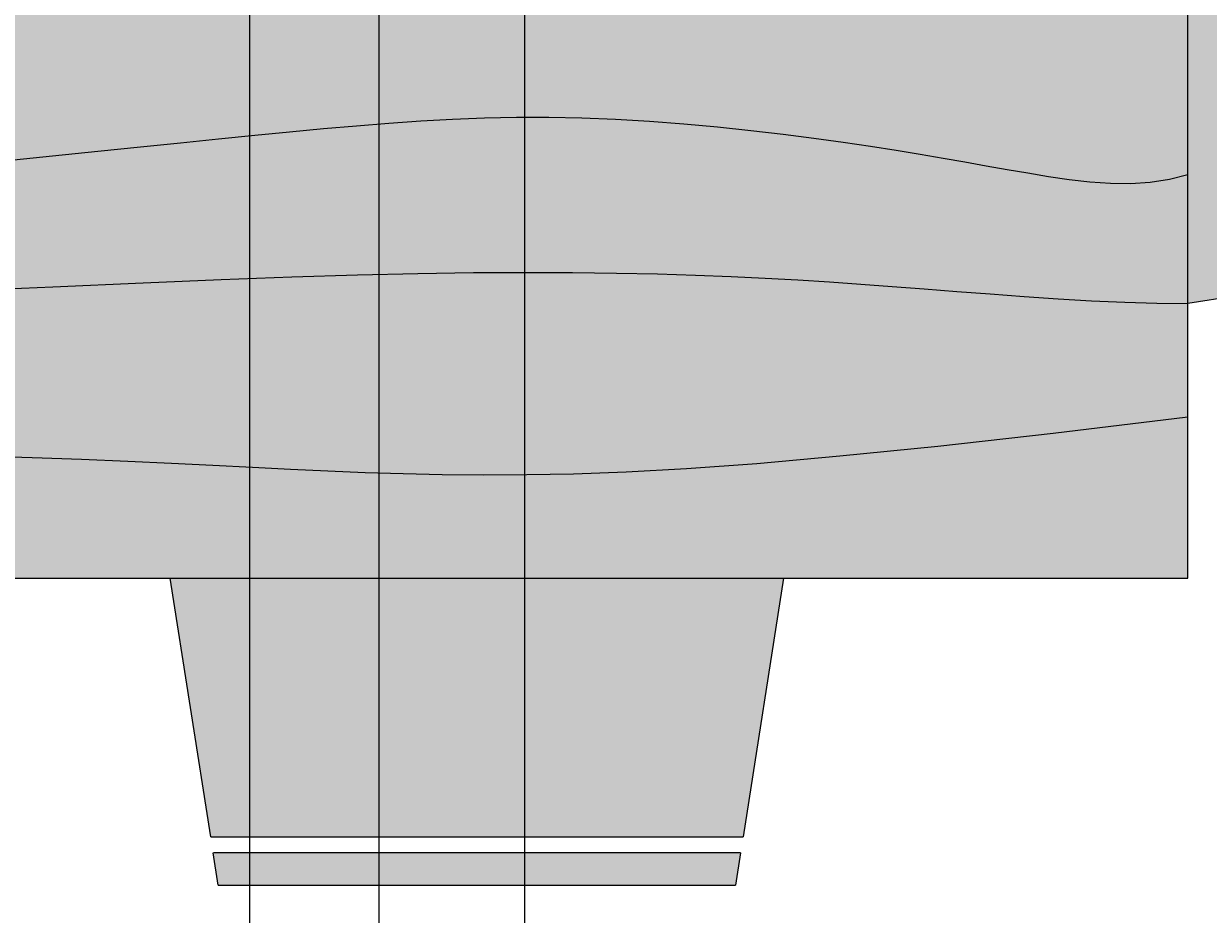
# Model space of a CAD drawing. Units: inches. Extents: x 1567 to 1964, y 1813 to 2447.
# Tile 19 of 28: x 1788 to 1825, y 2172 to 2199. Entities that reach past the tile are written whole.
import ezdxf

# ---------------------------------------------------------------- set-up
doc = ezdxf.new("R2010")
doc.units = ezdxf.units.IN
doc.layers.add('A-ANNO-DIMS', color=2, linetype='Continuous', lineweight=18)
doc.layers.add('A-FURN', color=8, linetype='Continuous', lineweight=18)
doc.layers.add('A-FURN-PATT', color=252, linetype='Continuous', lineweight=13, true_color=0x939598)
doc.styles.get("Standard").update_dxf_attribs({"font": 'arial.ttf'})
doc.dimstyles.get("Standard").update_dxf_attribs({"dimtxt": 0.18, "dimasz": 0.18, "dimexe": 0.18, "dimexo": 0.0625, "dimgap": 0.09, "dimtad": 0, "dimtih": 1, "dimtoh": 1, "dimdec": 4, "dimzin": 0, "dimdsep": 46, "dimtxsty": 'Standard', "dimcen": 0.09, "dimadec": 0, "dimazin": 0, "dimtfac": 1, "dimtdec": 4, "dimtofl": 0, "dimtmove": 0, "dimatfit": 3, "dimfxl": 1, "dimtolj": 1, "dimtzin": 0, "dimarcsym": 0})

# ---------------------------------------------------------------- blocks, each defined once
blk = doc.blocks.new('Dining Set - 36 x 72 in.')
for p, q in [((36, -18), (36, 18)), ((35.9976, -9.48476), (43.9993, -8.2345)), ((-36, -18), (36, -18)), ((5.7657, -26.0006), (4.5153, -17.99762)), ((23.4848, -17.99762), (22.2345, -25.99928)), ((5.7696, -26), (22.2392, -26)), ((6, -27.5), (5.8438, -26.50044)), ((22.1584, -26.5), (5.8466, -26.5)), ((22.1563, -26.49967), (22, -27.5)), ((6, -27.5), (22, -27.5))]:
    blk.add_line(p, q)
for points in [[(-0.625, -5.08334), (0.8708, -4.93099), (2.2715, -4.78646), (3.5872, -4.64974), (4.8281, -4.52084), (6.0046, -4.39974), (7.127, -4.28646), (8.2053, -4.18099), (9.25, -4.08334), (10.2705, -3.99382), (11.2734, -3.91407), (12.2647, -3.84603), (13.25, -3.79167), (14.2354, -3.75293), (15.2266, -3.73177), (16.2295, -3.73015), (17.25, -3.75), (18.2912, -3.79248), (19.3451, -3.85547), (20.4009, -3.93604), (21.4479, -4.03125), (22.4754, -4.13819), (23.4727, -4.25391), (24.4289, -4.37549), (25.3334, -4.5), (26.1785, -4.62492), (26.9694, -4.74935), (27.7145, -4.87281), (28.4219, -4.99479), (29.1, -5.11483), (29.7572, -5.23242), (30.4016, -5.34709), (31.0417, -5.45834), (31.6837, -5.56437), (32.3262, -5.65821), (32.9658, -5.73153), (33.599, -5.77604), (34.2224, -5.78345), (34.8327, -5.74545), (35.4264, -5.65373), (36, -5.5)], [(-2.5226, -9.12354), (0.8789, -8.98047), (3.6769, -8.85498), (6.0833, -8.75), (8.2767, -8.66765), (10.3021, -8.60677), (12.1712, -8.56543), (13.8958, -8.54167), (15.4876, -8.53353), (16.9583, -8.53907), (18.3197, -8.55632), (19.5834, -8.58334), (20.7616, -8.61841), (21.8685, -8.66081), (22.9188, -8.71004), (23.9271, -8.76563), (24.9081, -8.82707), (25.8763, -8.89388), (26.8465, -8.96558), (27.8334, -9.04167), (28.8474, -9.12118), (29.8828, -9.20117), (30.93, -9.27824), (31.9792, -9.34896), (33.0205, -9.40991), (34.0443, -9.45768), (35.0407, -9.48885), (36, -9.5)], [(-1.3709, -14.20785), (0.2448, -14.26042), (1.7647, -14.3169), (3.1973, -14.3763), (4.5507, -14.43767), (5.8333, -14.5), (7.0554, -14.5621), (8.235, -14.62175), (9.3922, -14.67652), (10.5469, -14.72396), (11.7192, -14.76164), (12.929, -14.78711), (14.1965, -14.79794), (15.5417, -14.79167), (16.9933, -14.76424), (18.6152, -14.70508), (20.4804, -14.60197), (22.6615, -14.44271), (25.2312, -14.21509), (28.2624, -13.9069), (31.8277, -13.50594), (36, -13)]]:
    blk.add_lwpolyline(points)
blk = doc.blocks.new('*D27')
at = {"layer": 'A-ANNO-DIMS', "color": 0, "lineweight": -2, "transparency": 16777216}
for p, q in [((1742.951, 2172.357), (1742.951, 2158.59)), ((1833.951, 2172.357), (1833.951, 2158.59)), ((1743.131, 2158.77), (1787.5, 2158.77)), ((1833.771, 2158.77), (1789.403, 2158.77))]:
    blk.add_line(p, q, dxfattribs=at)
at = {"layer": 'A-ANNO-DIMS', "color": 0, "transparency": 16777216}
for points in [[(1743.131, 2158.8), (1743.131, 2158.74), (1742.951, 2158.77)], [(1833.771, 2158.8), (1833.771, 2158.74), (1833.951, 2158.77)]]:
    blk.add_solid(points, dxfattribs=at)
at = {"layer": 'Defpoints', "color": 0, "transparency": 16777216}
for p in [(1742.951, 2172.42), (1833.951, 2172.42), (1833.951, 2158.77)]:
    blk.add_point(p, dxfattribs=at)
at = {"layer": 'A-ANNO-DIMS', "color": 0, "transparency": 16777216, "insert": (1788.451, 2158.77), "char_height": 0.18, "attachment_point": 5}
blk.add_mtext('\\A1;DINING SET 91', dxfattribs=at)
blk = doc.blocks.new('*D54')
at = {"layer": 'A-ANNO-DIMS', "color": 0, "lineweight": -2, "transparency": 16777216}
for p, q in [((1711.43, 1964.352), (1711.43, 2447.12)), ((1711.61, 2446.94), (1753.211, 2446.94)), ((1795.25, 2446.94), (1753.648, 2446.94)), ((1795.43, 1964.352), (1795.43, 2447.12))]:
    blk.add_line(p, q, dxfattribs=at)
at = {"layer": 'A-ANNO-DIMS', "color": 0, "transparency": 16777216}
for points in [[(1711.61, 2446.97), (1711.61, 2446.91), (1711.43, 2446.94)], [(1795.25, 2446.97), (1795.25, 2446.91), (1795.43, 2446.94)]]:
    blk.add_solid(points, dxfattribs=at)
at = {"layer": 'Defpoints', "color": 0, "transparency": 16777216}
for p in [(1795.43, 2446.94), (1711.43, 1964.29), (1795.43, 1964.29)]:
    blk.add_point(p, dxfattribs=at)
at = {"layer": 'A-ANNO-DIMS', "color": 0, "transparency": 16777216, "insert": (1753.43, 2446.94), "char_height": 0.18, "attachment_point": 5}
blk.add_mtext('\\A1;84', dxfattribs=at)
blk = doc.blocks.new('*D55')
at = {"layer": 'A-ANNO-DIMS', "color": 0, "lineweight": -2, "transparency": 16777216}
for p, q in [((1795.43, 1964.352), (1795.43, 2447.12)), ((1795.61, 2446.94), (1797.277, 2446.94)), ((1799.25, 2446.94), (1797.582, 2446.94)), ((1799.43, 1967.352), (1799.43, 2447.12))]:
    blk.add_line(p, q, dxfattribs=at)
at = {"layer": 'A-ANNO-DIMS', "color": 0, "transparency": 16777216}
for points in [[(1795.61, 2446.97), (1795.61, 2446.91), (1795.43, 2446.94)], [(1799.25, 2446.97), (1799.25, 2446.91), (1799.43, 2446.94)]]:
    blk.add_solid(points, dxfattribs=at)
at = {"layer": 'Defpoints', "color": 0, "transparency": 16777216}
for p in [(1799.43, 2446.94), (1799.43, 1967.29), (1795.43, 1964.29)]:
    blk.add_point(p, dxfattribs=at)
at = {"layer": 'A-ANNO-DIMS', "color": 0, "transparency": 16777216, "insert": (1797.43, 2446.94), "char_height": 0.18, "attachment_point": 5}
blk.add_mtext('\\A1;4', dxfattribs=at)
blk = doc.blocks.new('*D70')
at = {"layer": 'A-ANNO-DIMS', "color": 0, "lineweight": -2, "transparency": 16777216}
for p, q in [((1799.43, 1967.352), (1799.43, 2447.12)), ((1799.61, 2446.94), (1801.421, 2446.94)), ((1803.75, 2446.94), (1801.938, 2446.94)), ((1803.93, 1967.352), (1803.93, 2447.12))]:
    blk.add_line(p, q, dxfattribs=at)
at = {"layer": 'A-ANNO-DIMS', "color": 0, "transparency": 16777216}
for points in [[(1799.61, 2446.97), (1799.61, 2446.91), (1799.43, 2446.94)], [(1803.75, 2446.97), (1803.75, 2446.91), (1803.93, 2446.94)]]:
    blk.add_solid(points, dxfattribs=at)
at = {"layer": 'Defpoints', "color": 0, "transparency": 16777216}
for p in [(1803.93, 2446.94), (1799.43, 1967.29), (1803.93, 1967.29)]:
    blk.add_point(p, dxfattribs=at)
at = {"layer": 'A-ANNO-DIMS', "color": 0, "transparency": 16777216, "insert": (1801.68, 2446.94), "char_height": 0.18, "attachment_point": 5}
blk.add_mtext('\\A1;4.5', dxfattribs=at)
blk = doc.blocks.new('*D71')
at = {"layer": 'A-ANNO-DIMS', "color": 0, "lineweight": -2, "transparency": 16777216}
for p, q in [((1799.43, 1910.752), (1799.43, 2447.12)), ((1799.61, 2446.94), (1861.648, 2446.94)), ((1924.25, 2446.94), (1862.211, 2446.94)), ((1924.43, 1910.752), (1924.43, 2447.12))]:
    blk.add_line(p, q, dxfattribs=at)
at = {"layer": 'A-ANNO-DIMS', "color": 0, "transparency": 16777216}
for points in [[(1799.61, 2446.97), (1799.61, 2446.91), (1799.43, 2446.94)], [(1924.25, 2446.97), (1924.25, 2446.91), (1924.43, 2446.94)]]:
    blk.add_solid(points, dxfattribs=at)
at = {"layer": 'Defpoints', "color": 0, "transparency": 16777216}
for p in [(1924.43, 2446.94), (1799.43, 1910.69), (1924.43, 1910.69)]:
    blk.add_point(p, dxfattribs=at)
at = {"layer": 'A-ANNO-DIMS', "color": 0, "transparency": 16777216, "insert": (1861.93, 2446.94), "char_height": 0.18, "attachment_point": 5}
blk.add_mtext('\\A1;125', dxfattribs=at)

msp = doc.modelspace()

# ---------------------------------------------------------------- hatches: boundary and pattern name
at = {"layer": 'A-FURN-PATT'}
h = msp.add_hatch(color=256, dxfattribs=at)
h.dxf.hatch_style = 1
h.paths.add_polyline_path([(1621.2532, 2242.0229), (1643.7811, 2241.7239), (1643.8607, 2247.7234), (1617.863, 2248.0685, 0.1904762), (1616.7481, 2164.0759), (1642.7458, 2163.7308), (1642.8254, 2169.7302), (1620.2975, 2170.0293, -0.1519478)])
h.paths.add_polyline_path([(1673.5306, 2249.6607), (1653.8509, 2249.6607), (1653.8509, 2248.5031, 0.1176471), (1673.5306, 2248.5031)])
h.paths.add_polyline_path([(1706.0889, 2249.6607), (1686.4092, 2249.6607), (1686.4092, 2248.5031, 0.1176471), (1706.0889, 2248.5031)])
h.paths.add_polyline_path([(1782.4511, 2227.4197), (1766.4511, 2227.4197), (1766.2949, 2226.4197), (1782.6074, 2226.4197)])
h.paths.add_polyline_path([(1810.4511, 2227.4197), (1794.4511, 2227.4197), (1794.2949, 2226.4197), (1810.6074, 2226.4197)])
h.paths.add_polyline_path([(1743.9511, 2208.076), (1742.9511, 2207.9197), (1742.9511, 2191.9197), (1743.9511, 2191.7635)])
h.paths.add_polyline_path([(1782.6074, 2173.4197), (1766.2949, 2173.4197), (1766.4511, 2172.4197), (1782.4511, 2172.4197)])
h.paths.add_polyline_path([(1810.6074, 2173.4197), (1794.2949, 2173.4197), (1794.4511, 2172.4197), (1810.4511, 2172.4197)])
h.paths.add_polyline_path([(1861.053, 2006.5071), (1845.8531, 2006.5071), (1861.053, 1991.3071)])
h.paths.add_polyline_path([(1905.853, 1993.7071), (1861.053, 1993.7071), (1861.053, 1991.3071), (1905.853, 1991.3071)])
h.paths.add_polyline_path([(1919.7245, 2257.29, 0.5000001), (1918.7245, 2258.29), (1901.7245, 2258.29, 0.5000001), (1900.7245, 2257.29), (1900.7245, 2253.29, 0.5000001), (1901.7245, 2252.29), (1918.7245, 2252.29, 0.5000001), (1919.7245, 2253.29)])
h.paths.add_polyline_path([(1875.9094, 2391.0204), (1875.9094, 2375.8204), (1891.1093, 2375.8204)], flags=17)
h.paths.add_polyline_path([(1891.1093, 2405.4204), (1831.1094, 2405.4204), (1831.1094, 2391.0204), (1839.1093, 2391.0204), (1839.1093, 2404.2204), (1859.9093, 2404.2204), (1859.9093, 2391.0204), (1862.3093, 2391.0204), (1862.3093, 2404.2204), (1883.1093, 2404.2204), (1883.1093, 2389.0204), (1877.9094, 2389.0204), (1891.1093, 2375.8204)])
h.paths.add_polyline_path([(1682.1402, 2390.0316), (1682.1402, 2374.8316), (1697.3402, 2374.8316)], flags=17)
h.paths.add_polyline_path([(1697.3402, 2404.4316), (1637.3402, 2404.4316), (1637.3402, 2390.0316), (1645.3402, 2390.0316), (1645.3402, 2403.2316), (1666.1402, 2403.2316), (1666.1402, 2390.0316), (1668.5402, 2390.0316), (1668.5402, 2403.2316), (1689.3402, 2403.2316), (1689.3402, 2388.0316), (1684.1402, 2388.0316), (1697.3402, 2374.8316)])
h = msp.add_hatch(color=256, dxfattribs=at)
h.dxf.hatch_style = 1
h.paths.add_polyline_path([(1697.3402, 2374.8316), (1682.1402, 2374.8316), (1682.1402, 2387.6316), (1637.3402, 2387.6316), (1637.3402, 2324.4315), (1697.3402, 2324.4315)])
h.paths.add_polyline_path([(1891.1093, 2375.8204), (1875.9094, 2375.8204), (1875.9094, 2388.6204), (1831.1094, 2388.6204), (1831.1094, 2325.4204), (1891.1093, 2325.4204)])
h.paths.add_polyline_path([(1702.5611, 2206.8057), (1702.5611, 2210.8057), (1699.7395, 2209.9436), (1697.013, 2209.2403), (1694.3857, 2208.6763), (1691.8615, 2208.2326), (1689.4443, 2207.8896), (1687.1381, 2207.6282), (1684.9469, 2207.4289), (1682.8747, 2207.2725), (1680.9233, 2207.1425), (1679.0865, 2207.0339), (1677.3558, 2206.9445), (1675.7229, 2206.8719), (1674.1794, 2206.8141), (1672.7169, 2206.7688), (1671.327, 2206.7339), (1670.0014, 2206.707), (1668.7314, 2206.6866), (1667.5072, 2206.6732), (1666.3188, 2206.668), (1665.1561, 2206.6722), (1664.009, 2206.6869), (1662.8675, 2206.7133), (1661.7215, 2206.7525), (1660.5611, 2206.8057), (1660.5611, 2202.8057), (1661.9932, 2202.9556), (1663.3314, 2203.0744), (1664.5899, 2203.1671), (1665.7831, 2203.2385), (1666.9254, 2203.2935), (1668.0311, 2203.3368), (1669.1145, 2203.3734), (1670.1902, 2203.4081), (1671.2724, 2203.4451), (1672.3759, 2203.4866), (1673.5155, 2203.534), (1674.706, 2203.5887), (1675.9621, 2203.6523), (1677.2986, 2203.7262), (1678.7304, 2203.8118), (1680.2722, 2203.9108), (1681.947, 2204.0272), (1683.8108, 2204.1769), (1685.9279, 2204.3782), (1688.3626, 2204.6496), (1691.179, 2205.0096), (1694.4413, 2205.4767), (1698.214, 2206.0692)])
h.paths.add_polyline_path([(1702.5611, 2218.8057), (1701.9821, 2217.9383), (1701.3316, 2217.191), (1700.6091, 2216.5515), (1699.8141, 2216.0071), (1698.946, 2215.5454), (1698.0041, 2215.1536), (1696.9879, 2214.8194), (1695.8969, 2214.5301), (1694.7328, 2214.2753), (1693.5072, 2214.0522), (1692.2339, 2213.8602), (1690.9266, 2213.6989), (1689.5994, 2213.5675), (1688.266, 2213.4654), (1686.9402, 2213.392), (1685.636, 2213.3467), (1684.3619, 2213.3287), (1683.1053, 2213.3361), (1681.8482, 2213.3668), (1680.5727, 2213.4187), (1679.2608, 2213.4898), (1677.8948, 2213.5779), (1676.4565, 2213.6811), (1674.9282, 2213.7971), (1673.2982, 2213.9236), (1671.5804, 2214.0573), (1669.795, 2214.1945), (1667.9622, 2214.3316), (1666.1022, 2214.4649), (1664.2352, 2214.5908), (1662.3814, 2214.7056), (1660.5611, 2214.8057), (1660.5611, 2206.8057), (1661.7215, 2206.7525), (1662.8675, 2206.7133), (1664.009, 2206.6869), (1665.1561, 2206.6722), (1666.3188, 2206.668), (1667.5072, 2206.6732), (1668.7314, 2206.6866), (1670.0014, 2206.707), (1671.327, 2206.7339), (1672.7169, 2206.7688), (1674.1794, 2206.8141), (1675.7229, 2206.8719), (1677.3558, 2206.9445), (1679.0865, 2207.0339), (1680.9233, 2207.1425), (1682.8747, 2207.2725), (1684.9469, 2207.4289), (1687.1381, 2207.6282), (1689.4443, 2207.8896), (1691.8615, 2208.2326), (1694.3857, 2208.6763), (1697.013, 2209.2403), (1699.7395, 2209.9436), (1702.5611, 2210.8057)])
h.paths.add_polyline_path([(1700.6091, 2216.5515), (1701.3316, 2217.191), (1701.9821, 2217.9383), (1702.5611, 2218.8057), (1702.5611, 2222.8057), (1689.452, 2222.8057), (1689.0171, 2222.4556), (1688.4521, 2222.0354), (1687.7806, 2221.5662), (1687.0235, 2221.067), (1686.2019, 2220.5566), (1685.3367, 2220.0541), (1684.4491, 2219.5785), (1683.56, 2219.1486), (1682.6867, 2218.7795), (1681.8312, 2218.4692), (1680.9918, 2218.212), (1680.1667, 2218.0019), (1679.3541, 2217.833), (1678.5524, 2217.6995), (1677.7597, 2217.5954), (1676.9744, 2217.5149), (1676.1942, 2217.4531), (1675.4146, 2217.4093), (1674.6309, 2217.384), (1673.8381, 2217.3774), (1673.0313, 2217.39), (1672.2056, 2217.4221), (1671.3562, 2217.4741), (1670.4782, 2217.5463), (1669.5642, 2217.639), (1668.5968, 2217.7516), (1667.5562, 2217.8833), (1666.4226, 2218.0336), (1665.1761, 2218.2017), (1663.7969, 2218.3869), (1662.2651, 2218.5885), (1660.5611, 2218.8057), (1660.5611, 2214.8057), (1662.3814, 2214.7056), (1664.2352, 2214.5908), (1666.1022, 2214.4649), (1667.9622, 2214.3316), (1669.795, 2214.1945), (1671.5804, 2214.0573), (1673.2982, 2213.9236), (1674.9282, 2213.7971), (1676.4565, 2213.6811), (1677.8948, 2213.5779), (1679.2608, 2213.4898), (1680.5727, 2213.4187), (1681.8482, 2213.3668), (1683.1053, 2213.3361), (1684.3619, 2213.3287), (1685.636, 2213.3467), (1686.9402, 2213.392), (1688.266, 2213.4654), (1689.5994, 2213.5675), (1690.9266, 2213.6989), (1692.2339, 2213.8602), (1693.5072, 2214.0522), (1694.7328, 2214.2753), (1695.8969, 2214.5301), (1696.9879, 2214.8194), (1698.0041, 2215.1536), (1698.946, 2215.5454), (1699.8141, 2216.0071)])
h.paths.add_polyline_path([(1687.0235, 2221.067), (1687.7806, 2221.5662), (1688.4521, 2222.0354), (1689.0171, 2222.4556), (1689.452, 2222.8057), (1660.5611, 2222.8057), (1660.5611, 2218.8057), (1662.2651, 2218.5885), (1663.7969, 2218.3869), (1665.1761, 2218.2017), (1666.4226, 2218.0336), (1667.5562, 2217.8833), (1668.5968, 2217.7516), (1669.5642, 2217.639), (1670.4782, 2217.5463), (1671.3562, 2217.4741), (1672.2056, 2217.4221), (1673.0313, 2217.39), (1673.8381, 2217.3774), (1674.6309, 2217.384), (1675.4146, 2217.4093), (1676.1942, 2217.4531), (1676.9744, 2217.5149), (1677.7597, 2217.5954), (1678.5524, 2217.6995), (1679.3541, 2217.833), (1680.1667, 2218.0019), (1680.9918, 2218.212), (1681.8312, 2218.4692), (1682.6867, 2218.7795), (1683.56, 2219.1486), (1684.4491, 2219.5785), (1685.3367, 2220.0541), (1686.2019, 2220.5566)], flags=17)
h.paths.add_polyline_path([(1702.5611, 2198.8057), (1698.9289, 2199.2412), (1695.8472, 2199.5774), (1693.2166, 2199.8257), (1690.9377, 2199.9973), (1688.9111, 2200.1033), (1687.0375, 2200.155), (1685.2174, 2200.1637), (1683.3514, 2200.1406), (1681.3514, 2200.0941), (1679.1736, 2200.0225), (1676.7858, 2199.921), (1674.1554, 2199.7852), (1671.2502, 2199.6103), (1668.0377, 2199.3919), (1664.4854, 2199.1252), (1660.5611, 2198.8057), (1660.5611, 2194.8057), (1662.2697, 2194.9771), (1663.9673, 2195.0999), (1665.6339, 2195.1809), (1667.2495, 2195.227), (1668.7941, 2195.2449), (1670.2478, 2195.2414), (1671.5906, 2195.2233), (1672.8026, 2195.1974), (1673.8739, 2195.1689), (1674.8359, 2195.1364), (1675.7302, 2195.0967), (1676.5982, 2195.0469), (1677.4817, 2194.9838), (1678.422, 2194.9043), (1679.4609, 2194.8055), (1680.6397, 2194.6842), (1682.005, 2194.5341), (1683.6223, 2194.335), (1685.562, 2194.0637), (1687.8945, 2193.6967), (1690.6902, 2193.2108), (1694.0196, 2192.5826), (1697.9531, 2191.7887), (1702.5611, 2190.8057)])
h.paths.add_polyline_path([(1702.5611, 2206.8057), (1698.214, 2206.0692), (1694.4413, 2205.4767), (1691.179, 2205.0096), (1688.3626, 2204.6496), (1685.9279, 2204.3782), (1683.8108, 2204.1769), (1681.947, 2204.0272), (1680.2722, 2203.9108), (1678.7304, 2203.8118), (1677.2986, 2203.7262), (1675.9621, 2203.6523), (1674.706, 2203.5887), (1673.5155, 2203.534), (1672.3759, 2203.4866), (1671.2724, 2203.4451), (1670.1902, 2203.4081), (1669.1145, 2203.3734), (1668.0311, 2203.3368), (1666.9254, 2203.2935), (1665.7831, 2203.2385), (1664.5899, 2203.1671), (1663.3314, 2203.0744), (1661.9932, 2202.9556), (1660.5611, 2202.8057), (1660.5611, 2198.8057), (1664.4854, 2199.1252), (1668.0377, 2199.3919), (1671.2502, 2199.6103), (1674.1554, 2199.7852), (1676.7858, 2199.921), (1679.1736, 2200.0225), (1681.3514, 2200.0941), (1683.3514, 2200.1406), (1685.2174, 2200.1637), (1687.0375, 2200.155), (1688.9111, 2200.1033), (1690.9377, 2199.9973), (1693.2166, 2199.8257), (1695.8472, 2199.5774), (1698.9289, 2199.2412), (1702.5611, 2198.8057)])
h.paths.add_polyline_path([(1702.5611, 2190.8057), (1697.9531, 2191.7887), (1694.0196, 2192.5826), (1690.6902, 2193.2108), (1687.8945, 2193.6967), (1685.562, 2194.0637), (1683.6223, 2194.335), (1682.005, 2194.5341), (1680.6397, 2194.6842), (1679.4609, 2194.8055), (1678.422, 2194.9043), (1677.4817, 2194.9838), (1676.5982, 2195.0469), (1675.7302, 2195.0967), (1674.8359, 2195.1364), (1673.8739, 2195.1689), (1672.8026, 2195.1974), (1671.5906, 2195.2233), (1670.2478, 2195.2414), (1668.7941, 2195.2449), (1667.2495, 2195.227), (1665.6339, 2195.1809), (1663.9673, 2195.0999), (1662.2697, 2194.9771), (1660.5611, 2194.8057), (1660.5611, 2190.8057), (1665.9637, 2190.2699), (1670.5105, 2189.7867), (1674.3035, 2189.3504), (1677.4445, 2188.9552), (1680.0354, 2188.5951), (1682.1782, 2188.2644), (1683.9747, 2187.9571), (1685.5268, 2187.6675), (1686.9225, 2187.3901), (1688.1943, 2187.1216), (1689.3606, 2186.859), (1690.4399, 2186.5993), (1691.4508, 2186.3396), (1692.4118, 2186.0769), (1693.3413, 2185.8084), (1694.2579, 2185.531), (1695.1786, 2185.2422), (1696.1142, 2184.9406), (1697.0739, 2184.6252), (1698.0671, 2184.2949), (1699.1032, 2183.9489), (1700.1913, 2183.586), (1701.3408, 2183.2053), (1702.5611, 2182.8057)])
h.paths.add_polyline_path([(1702.5611, 2182.8057), (1701.3408, 2183.2053), (1700.1913, 2183.586), (1699.1032, 2183.9489), (1698.0671, 2184.2949), (1697.0739, 2184.6252), (1696.1142, 2184.9406), (1695.1786, 2185.2422), (1694.2579, 2185.531), (1693.3413, 2185.8084), (1692.4118, 2186.0769), (1691.4508, 2186.3396), (1690.4399, 2186.5993), (1689.3606, 2186.859), (1688.1943, 2187.1216), (1686.9225, 2187.3901), (1685.5268, 2187.6675), (1683.9747, 2187.9571), (1682.1782, 2188.2644), (1680.0354, 2188.5951), (1677.4445, 2188.9552), (1674.3035, 2189.3504), (1670.5105, 2189.7867), (1665.9637, 2190.2699), (1660.5611, 2190.8057), (1660.5611, 2186.8057), (1663.5709, 2186.52), (1666.0965, 2186.2414), (1668.1979, 2185.9698), (1669.9351, 2185.7048), (1671.3681, 2185.446), (1672.5568, 2185.1931), (1673.5613, 2184.9458), (1674.4415, 2184.7037), (1675.2485, 2184.4664), (1675.9976, 2184.2328), (1677.0295, 2183.8907), (1678.2492, 2183.4332), (1679.354, 2182.9669), (1680.4123, 2182.4724), (1681.3757, 2181.9718), (1682.2435, 2181.4594), (1683.1864, 2180.8057), (1702.5611, 2180.8057)])
h.paths.add_polyline_path([(1677.3469, 2183.7716), (1676.6949, 2184.0016), (1675.9976, 2184.2328), (1675.2485, 2184.4664), (1674.4415, 2184.7037), (1673.5613, 2184.9458), (1672.5568, 2185.1931), (1671.3681, 2185.446), (1669.9351, 2185.7048), (1668.1979, 2185.9698), (1666.0965, 2186.2414), (1663.5709, 2186.52), (1660.5611, 2186.8057), (1660.5611, 2180.8057), (1683.1506, 2180.8057), (1682.802, 2181.0722), (1682.4264, 2181.3326), (1682.0201, 2181.5913), (1681.586, 2181.8476), (1681.1268, 2182.1011), (1680.6453, 2182.3513), (1680.1443, 2182.5976), (1679.6266, 2182.8395), (1679.0933, 2183.0769), (1678.5398, 2183.3105), (1677.9598, 2183.5417)], flags=17)
h.paths.add_polyline_path([(1824.4511, 2199.9016), (1824.089, 2199.9302), (1824.0595, 2199.9372), (1824.0397, 2199.9406), (1823.5413, 2200.0576), (1823.4095, 2200.0864), (1823.0664, 2200.1559), (1822.6419, 2200.2361), (1822.1519, 2200.3222), (1821.6126, 2200.4093), (1821.0401, 2200.4925), (1820.4505, 2200.5669), (1819.8599, 2200.6276), (1819.2845, 2200.6697), (1818.7366, 2200.6896), (1818.2141, 2200.688), (1817.7112, 2200.6668), (1817.222, 2200.6281), (1816.7405, 2200.5737), (1816.261, 2200.5057), (1815.7776, 2200.4259), (1815.2845, 2200.3364), (1814.3007, 2200.149), (1813.3315, 2199.9765), (1812.406, 2199.8514), (1811.6868, 2199.7739), (1810.8992, 2199.7121), (1810.0345, 2199.6697), (1809.0854, 2199.6497), (1808.0514, 2199.6502), (1806.9334, 2199.6683), (1805.7324, 2199.701), (1804.4493, 2199.7454), (1803.0852, 2199.7986), (1801.641, 2199.8577), (1800.1178, 2199.9197), (1798.5134, 2199.9818), (1796.8144, 2200.0415), (1795.004, 2200.0962), (1793.0657, 2200.1437), (1790.9828, 2200.1814), (1788.7389, 2200.2068), (1786.3171, 2200.2177), (1783.7011, 2200.2114), (1780.8715, 2200.185), (1777.7988, 2200.1326), (1774.4506, 2200.0481), (1770.7948, 2199.9249), (1766.7992, 2199.7569), (1762.4316, 2199.5376), (1757.6596, 2199.2606), (1752.4511, 2198.9197), (1752.4511, 2193.4197), (1761.2668, 2193.6071), (1768.3671, 2193.7934), (1773.9821, 2193.9778), (1778.3417, 2194.1593), (1781.6759, 2194.3369), (1784.2148, 2194.5096), (1786.1882, 2194.6764), (1787.8261, 2194.8364), (1789.3219, 2194.9887), (1790.7226, 2195.1333), (1792.0383, 2195.27), (1793.2792, 2195.3989), (1794.4557, 2195.52), (1795.5781, 2195.6333), (1796.6564, 2195.7387), (1797.7011, 2195.8364), (1798.7216, 2195.9259), (1799.7245, 2196.0057), (1800.7158, 2196.0737), (1801.7011, 2196.1281), (1802.6865, 2196.1668), (1803.6777, 2196.188), (1804.6806, 2196.1896), (1805.7011, 2196.1697), (1806.7423, 2196.1273), (1807.7962, 2196.0643), (1808.852, 2195.9837), (1809.899, 2195.8885), (1810.9265, 2195.7815), (1811.9238, 2195.6658), (1812.88, 2195.5442), (1813.7845, 2195.4197), (1814.6296, 2195.2948), (1815.4205, 2195.1704), (1816.1656, 2195.0469), (1816.873, 2194.9249), (1817.5511, 2194.8049), (1818.2083, 2194.6873), (1818.8527, 2194.5726), (1819.4928, 2194.4614), (1820.1348, 2194.3554), (1820.7773, 2194.2615), (1821.4169, 2194.1882), (1822.0501, 2194.1437), (1822.6735, 2194.1363), (1823.2838, 2194.1743), (1823.8775, 2194.266), (1824.4511, 2194.4197)])
h.paths.add_polyline_path([(1821.4716, 2190.5098), (1820.4303, 2190.5708), (1819.3811, 2190.6415), (1818.3339, 2190.7186), (1817.2985, 2190.7986), (1816.2845, 2190.8781), (1815.2976, 2190.9542), (1814.3274, 2191.0259), (1813.3592, 2191.0927), (1812.3782, 2191.1541), (1811.3699, 2191.2097), (1810.3196, 2191.2589), (1809.2127, 2191.3013), (1808.0345, 2191.3364), (1806.7708, 2191.3634), (1805.4094, 2191.3807), (1803.9387, 2191.3862), (1802.3469, 2191.3781), (1800.6223, 2191.3543), (1798.7532, 2191.313), (1796.7278, 2191.2521), (1794.5344, 2191.1697), (1792.128, 2191.0648), (1789.33, 2190.9393), (1785.9285, 2190.7962), (1781.7115, 2190.6385), (1776.4672, 2190.469), (1769.9836, 2190.2908), (1762.0489, 2190.1067), (1752.4511, 2189.9197), (1752.4511, 2185.4197), (1758.363, 2185.5846), (1763.4179, 2185.7075), (1767.7199, 2185.7933), (1771.373, 2185.8468), (1774.4811, 2185.873), (1777.1484, 2185.8768), (1779.4787, 2185.8629), (1781.5761, 2185.8364), (1783.5287, 2185.8014), (1785.3606, 2185.7596), (1787.0802, 2185.7119), (1788.6959, 2185.6593), (1790.2158, 2185.6028), (1791.6484, 2185.5434), (1793.0018, 2185.4821), (1794.2844, 2185.4197), (1795.5065, 2185.3576), (1796.6861, 2185.298), (1797.8433, 2185.2432), (1798.998, 2185.1958), (1800.1703, 2185.1581), (1801.3801, 2185.1326), (1802.6476, 2185.1218), (1803.9928, 2185.1281), (1805.4444, 2185.1555), (1807.0663, 2185.2147), (1808.9315, 2185.3178), (1811.1126, 2185.477), (1813.6823, 2185.7046), (1816.7135, 2186.0128), (1820.2788, 2186.4138), (1824.4511, 2186.9197), (1824.4511, 2190.4197), (1823.4918, 2190.4309), (1822.4954, 2190.4621)])
h.paths.add_polyline_path([(1797.3762, 2216.0584), (1797.6199, 2216.2267), (1797.9558, 2216.3355), (1798.3017, 2216.3703), (1798.5761, 2216.3781), (1798.8974, 2216.3703), (1799.2714, 2216.3468), (1799.704, 2216.3078), (1800.2011, 2216.2531), (1800.7695, 2216.1829), (1801.4205, 2216.0981), (1802.1662, 2215.9996), (1803.0188, 2215.8885), (1803.9906, 2215.7656), (1805.0937, 2215.632), (1806.3404, 2215.4886), (1807.7428, 2215.3364), (1809.3101, 2215.1764), (1811.039, 2215.0096), (1812.9232, 2214.8369), (1814.9563, 2214.6593), (1817.132, 2214.4778), (1819.444, 2214.2934), (1821.8858, 2214.1071), (1824.4511, 2213.9197), (1824.4511, 2217.9197), (1752.4511, 2217.9197), (1752.4511, 2214.9197), (1757.2739, 2214.8973), (1761.6432, 2214.8338), (1765.5973, 2214.7352), (1769.1751, 2214.6072), (1772.4149, 2214.4559), (1775.3554, 2214.2869), (1778.0352, 2214.1063), (1780.4928, 2213.9197), (1782.7607, 2213.7329), (1784.8476, 2213.5499), (1786.7557, 2213.3748), (1788.4876, 2213.2114), (1790.0456, 2213.0636), (1791.4322, 2212.9354), (1792.6499, 2212.8305), (1793.7011, 2212.7531), (1794.5904, 2212.7059), (1795.3313, 2212.688), (1795.9394, 2212.6974), (1796.4303, 2212.7322), (1796.8196, 2212.7905), (1797.123, 2212.8703), (1797.356, 2212.9695), (1797.5344, 2213.0864), (1797.6716, 2213.2187), (1797.7727, 2213.3637), (1797.8406, 2213.5185), (1797.8782, 2213.6801), (1797.8884, 2213.8457), (1797.8743, 2214.0122), (1797.8386, 2214.1767), (1797.7844, 2214.3364), (1797.7149, 2214.4889), (1797.6347, 2214.6346), (1797.5486, 2214.7744), (1797.3327, 2215.109), (1797.178, 2215.4303), (1797.1896, 2215.7939)])
h.paths.add_polyline_path([(1804.7872, 2210.6789), (1804.546, 2211.022), (1804.3512, 2211.3917), (1804.2466, 2211.7546), (1804.2574, 2212.0998), (1804.4058, 2212.4178), (1804.7068, 2212.7007), (1805.1359, 2212.9124), (1805.5279, 2212.9926), (1805.8136, 2213.0154), (1806.1178, 2213.0031), (1806.4405, 2212.9529), (1806.7929, 2212.867), (1807.1893, 2212.7489), (1807.6438, 2212.602), (1808.1706, 2212.4297), (1808.7838, 2212.2355), (1809.4976, 2212.0227), (1810.3261, 2211.7947), (1811.2868, 2211.5533), (1812.4101, 2211.2928), (1813.7297, 2211.0059), (1815.2793, 2210.6854), (1817.0925, 2210.3238), (1819.2031, 2209.9139), (1821.6447, 2209.4483), (1824.4511, 2208.9197), (1824.4511, 2213.9197), (1821.8858, 2214.1071), (1819.444, 2214.2934), (1817.132, 2214.4778), (1814.9563, 2214.6593), (1812.9232, 2214.8369), (1811.039, 2215.0096), (1809.3101, 2215.1764), (1807.7428, 2215.3364), (1806.3404, 2215.4886), (1805.0937, 2215.632), (1803.9906, 2215.7656), (1803.0188, 2215.8885), (1802.1662, 2215.9996), (1801.4205, 2216.0981), (1800.7695, 2216.1829), (1800.2011, 2216.2531), (1799.704, 2216.3078), (1799.2714, 2216.3468), (1798.8974, 2216.3703), (1798.5761, 2216.3781), (1798.3017, 2216.3703), (1798.0683, 2216.3468), (1797.87, 2216.3078), (1797.7011, 2216.2531), (1797.5566, 2216.1831), (1797.4355, 2216.0994), (1797.3378, 2216.004), (1797.2636, 2215.8989), (1797.2128, 2215.7859), (1797.1855, 2215.6671), (1797.1816, 2215.5444), (1797.2011, 2215.4197), (1797.2433, 2215.2946), (1797.304, 2215.1684), (1797.3783, 2215.0403), (1797.4615, 2214.9093), (1797.6718, 2214.5836), (1797.8218, 2214.2545), (1797.8933, 2213.9247), (1797.8728, 2213.5918), (1797.7366, 2213.2814), (1797.4586, 2213.0132), (1797.123, 2212.8703), (1796.8196, 2212.7905), (1796.4303, 2212.7322), (1795.9394, 2212.6974), (1795.3313, 2212.688), (1794.5904, 2212.7059), (1793.7011, 2212.7531), (1792.6499, 2212.8305), (1791.4322, 2212.9354), (1790.0456, 2213.0636), (1788.4876, 2213.2114), (1786.7557, 2213.3748), (1784.8476, 2213.5499), (1782.7607, 2213.7329), (1780.4928, 2213.9197), (1778.0352, 2214.1063), (1775.3554, 2214.2869), (1772.4149, 2214.4559), (1769.1751, 2214.6072), (1765.5973, 2214.7352), (1761.6432, 2214.8338), (1757.2739, 2214.8973), (1752.4511, 2214.9197), (1752.4511, 2209.9197), (1759.4745, 2210.0625), (1765.2786, 2210.1242), (1770.027, 2210.1175), (1773.8834, 2210.0551), (1777.0112, 2209.9498), (1779.5741, 2209.8143), (1781.7357, 2209.6611), (1783.6594, 2209.5031), (1785.4813, 2209.3506), (1787.2265, 2209.2049), (1788.8926, 2209.0651), (1790.4771, 2208.9301), (1791.9777, 2208.7991), (1793.3919, 2208.671), (1794.7171, 2208.5449), (1795.9511, 2208.4197), (1797.0922, 2208.2952), (1798.1425, 2208.1736), (1799.1049, 2208.0579), (1799.9823, 2207.951), (1800.7778, 2207.8558), (1801.4941, 2207.7752), (1802.1342, 2207.7122), (1802.7011, 2207.6697), (1803.1982, 2207.65), (1803.6308, 2207.6528), (1804.0048, 2207.6771), (1804.3261, 2207.7218), (1804.6005, 2207.7861), (1804.8339, 2207.869), (1805.0322, 2207.9694), (1805.2011, 2208.0864), (1805.3455, 2208.2189), (1805.4654, 2208.365), (1805.56, 2208.5229), (1805.6282, 2208.6906), (1805.6691, 2208.866), (1805.6816, 2209.0473), (1805.6648, 2209.2326), (1805.6178, 2209.4197), (1805.5406, 2209.6072), (1805.4381, 2209.7947), (1805.316, 2209.9822), (1805.1803, 2210.1697), (1805.0367, 2210.3572)])
h.paths.add_polyline_path([(1801.4941, 2207.7752), (1800.7778, 2207.8558), (1799.9823, 2207.951), (1799.1049, 2208.0579), (1798.1425, 2208.1736), (1797.0922, 2208.2952), (1795.9511, 2208.4197), (1794.7171, 2208.5449), (1793.3919, 2208.671), (1791.9777, 2208.7991), (1790.4771, 2208.9301), (1788.8926, 2209.0651), (1787.2265, 2209.2049), (1785.4813, 2209.3506), (1783.6594, 2209.5031), (1781.7357, 2209.6611), (1779.5741, 2209.8143), (1777.0112, 2209.9498), (1773.8834, 2210.0551), (1770.027, 2210.1175), (1765.2786, 2210.1242), (1759.4745, 2210.0625), (1752.4511, 2209.9197), (1752.4511, 2205.4197), (1757.7354, 2205.2545), (1762.3821, 2205.1294), (1766.4565, 2205.0374), (1770.024, 2204.9718), (1773.1502, 2204.9258), (1775.9003, 2204.8924), (1778.3399, 2204.8649), (1780.5344, 2204.8364), (1782.5421, 2204.8014), (1784.3925, 2204.7596), (1786.1082, 2204.7119), (1787.7115, 2204.6593), (1789.225, 2204.6028), (1790.6711, 2204.5434), (1792.0724, 2204.4821), (1793.4511, 2204.4197), (1794.8241, 2204.3576), (1796.1855, 2204.2973), (1797.5234, 2204.241), (1798.8261, 2204.1906), (1800.082, 2204.1479), (1801.2792, 2204.115), (1802.4062, 2204.0939), (1803.4511, 2204.0864), (1804.4051, 2204.0942), (1805.2701, 2204.1176), (1806.0512, 2204.1567), (1806.7532, 2204.2114), (1807.381, 2204.2817), (1807.9394, 2204.3676), (1808.4334, 2204.4692), (1808.8678, 2204.5864), (1809.248, 2204.7187), (1809.5813, 2204.8637), (1809.8756, 2205.0185), (1810.1386, 2205.1801), (1810.3782, 2205.3457), (1810.6022, 2205.5122), (1810.9725, 2205.7941), (1811.3803, 2206.072), (1811.739, 2206.2612), (1812.0032, 2206.3781), (1812.2869, 2206.4793), (1812.5931, 2206.563), (1812.9246, 2206.6271), (1813.2845, 2206.6697), (1813.6746, 2206.6894), (1814.0931, 2206.6867), (1814.5369, 2206.6624), (1815.0032, 2206.6176), (1815.489, 2206.5534), (1815.9915, 2206.4705), (1816.5076, 2206.3701), (1817.0345, 2206.2531), (1817.5753, 2206.1196), (1818.1582, 2205.9666), (1818.8172, 2205.7902), (1819.5865, 2205.5864), (1820.5004, 2205.3514), (1821.5931, 2205.0812), (1822.8986, 2204.7719), (1824.4511, 2204.4197), (1824.4511, 2208.9197), (1821.6447, 2209.4483), (1819.2031, 2209.9139), (1817.0925, 2210.3238), (1815.2793, 2210.6854), (1813.7297, 2211.0059), (1812.4101, 2211.2928), (1811.2868, 2211.5533), (1810.3261, 2211.7947), (1809.4976, 2212.0227), (1808.7838, 2212.2355), (1808.1706, 2212.4297), (1807.6438, 2212.602), (1807.1893, 2212.7489), (1806.7929, 2212.867), (1806.4405, 2212.9529), (1806.1178, 2213.0031), (1805.8136, 2213.0154), (1805.5279, 2212.9926), (1805.2638, 2212.9386), (1805.024, 2212.8572), (1804.8116, 2212.7524), (1804.6295, 2212.6281), (1804.4806, 2212.4881), (1804.3678, 2212.3364), (1804.2931, 2212.1764), (1804.2545, 2212.0096), (1804.2491, 2211.8369), (1804.274, 2211.6593), (1804.3263, 2211.4778), (1804.4029, 2211.2934), (1804.5011, 2211.1071), (1804.6178, 2210.9197), (1804.7496, 2210.7322), (1804.8912, 2210.5447), (1805.154, 2210.2061), (1805.3962, 2209.8715), (1805.5964, 2209.5053), (1805.688, 2209.1402), (1805.6629, 2208.7758), (1805.5257, 2208.4385), (1805.2839, 2208.1437), (1804.9434, 2207.9078), (1804.6005, 2207.7861), (1804.3261, 2207.7218), (1804.0048, 2207.6771), (1803.6308, 2207.6528), (1803.1982, 2207.65), (1802.7011, 2207.6697), (1802.1342, 2207.7122)])
h.paths.add_polyline_path([(1824.4511, 2204.4197), (1822.8986, 2204.7719), (1821.5931, 2205.0812), (1820.5004, 2205.3514), (1819.5865, 2205.5864), (1818.8172, 2205.7902), (1818.1582, 2205.9666), (1817.5753, 2206.1196), (1817.0345, 2206.2531), (1816.5076, 2206.3701), (1815.9915, 2206.4705), (1815.489, 2206.5534), (1815.0032, 2206.6176), (1814.5369, 2206.6624), (1814.0931, 2206.6867), (1813.6746, 2206.6894), (1813.2845, 2206.6697), (1812.9246, 2206.6271), (1812.5931, 2206.563), (1812.2869, 2206.4793), (1812.0032, 2206.3781), (1811.739, 2206.2612), (1811.4915, 2206.1307), (1811.2576, 2205.9884), (1811.0345, 2205.8364), (1810.8183, 2205.6767), (1810.4357, 2205.3854), (1810.1386, 2205.1801), (1809.8756, 2205.0185), (1809.5813, 2204.8637), (1809.248, 2204.7187), (1808.8678, 2204.5864), (1808.4334, 2204.4692), (1807.9394, 2204.3676), (1807.381, 2204.2817), (1806.7532, 2204.2114), (1806.0512, 2204.1567), (1805.2701, 2204.1176), (1804.4051, 2204.0942), (1803.4511, 2204.0864), (1802.4062, 2204.0939), (1801.2792, 2204.115), (1800.082, 2204.1479), (1798.8261, 2204.1906), (1797.5234, 2204.241), (1796.1855, 2204.2973), (1794.8241, 2204.3576), (1793.4511, 2204.4197), (1792.0724, 2204.4821), (1790.6711, 2204.5434), (1789.225, 2204.6028), (1787.7115, 2204.6593), (1786.1082, 2204.7119), (1784.3925, 2204.7596), (1782.5421, 2204.8014), (1780.5344, 2204.8364), (1778.3399, 2204.8649), (1775.9003, 2204.8924), (1773.1502, 2204.9258), (1770.024, 2204.9718), (1766.4565, 2205.0374), (1762.3821, 2205.1294), (1757.7354, 2205.2545), (1752.4511, 2205.4197), (1752.4511, 2198.9197), (1757.6596, 2199.2606), (1762.4316, 2199.5376), (1766.7992, 2199.7569), (1770.7948, 2199.9249), (1774.4506, 2200.0481), (1777.7988, 2200.1326), (1780.8715, 2200.185), (1783.7011, 2200.2114), (1786.3171, 2200.2177), (1788.7389, 2200.2068), (1790.9828, 2200.1814), (1793.0657, 2200.1437), (1795.004, 2200.0962), (1796.8144, 2200.0415), (1798.5134, 2199.9818), (1800.1178, 2199.9197), (1801.641, 2199.8577), (1803.0852, 2199.7986), (1804.4493, 2199.7454), (1805.7324, 2199.701), (1806.9334, 2199.6683), (1808.0514, 2199.6502), (1809.0854, 2199.6497), (1810.0345, 2199.6697), (1810.8992, 2199.7121), (1811.6868, 2199.7739), (1812.406, 2199.8514), (1813.0657, 2199.9406), (1813.6746, 2200.0376), (1814.2415, 2200.1385), (1814.7752, 2200.2394), (1815.2845, 2200.3364), (1815.7776, 2200.4259), (1816.261, 2200.5057), (1816.7405, 2200.5737), (1817.222, 2200.6281), (1817.7112, 2200.6668), (1818.2141, 2200.688), (1818.7366, 2200.6896), (1819.2845, 2200.6697), (1819.8599, 2200.6276), (1820.4505, 2200.5669), (1821.0401, 2200.4925), (1821.6126, 2200.4093), (1822.1519, 2200.3222), (1822.6419, 2200.2361), (1823.0664, 2200.1559), (1823.5408, 2200.0598), (1824.0595, 2199.9372), (1824.1105, 2199.9285), (1824.1888, 2199.9223), (1824.2953, 2199.9201), (1824.4511, 2199.9197)])
h.paths.add_polyline_path([(1795.4295, 2021.5492), (1771.4295, 2021.5492), (1771.4295, 1988.29), (1735.4295, 1988.29), (1735.4295, 2055.79), (1711.4295, 2055.79), (1711.4295, 1964.29), (1795.4295, 1964.29)])
h.paths.add_polyline_path([(1681.4295, 2063.29), (1674.0411, 2043.4455), (1681.4295, 2043.4455), (1688.818, 2043.4455)])
h.paths.add_polyline_path([(1843.2327, 2065.967), (1919.26, 2065.967), (1919.26, 2095.8187), (1843.2327, 2095.8187)], flags=9)
h = msp.add_hatch(color=256, dxfattribs=at)
h.dxf.hatch_style = 1
h.paths.add_polyline_path([(1642.2233, 2241.7446), (1623.1648, 2241.9976), (1622.8462, 2217.9997), (1641.9047, 2217.7467)])
h.paths.add_polyline_path([(1641.9047, 2217.7467), (1622.8462, 2217.9997), (1622.5277, 2194.0018), (1641.5862, 2193.7488)])
h.paths.add_polyline_path([(1641.5862, 2193.7488), (1622.5277, 2194.0018), (1622.2091, 2170.0039), (1641.2677, 2169.7509)])
h.paths.add_polyline_path([(1671.2154, 2243.8726, -0.236068), (1673.5306, 2245.0302), (1673.5306, 2246.1879), (1653.8509, 2246.1879), (1653.8509, 2245.0302, -0.236068), (1656.1662, 2243.8726), (1656.1662, 2233.4539, -0.236068), (1653.8509, 2232.2963), (1653.8509, 2231.1387, 0.1176471), (1673.5306, 2231.1387), (1673.5306, 2232.2963, -0.236068), (1671.2154, 2233.4539)])
h.paths.add_polyline_path([(1703.7736, 2243.8726, -0.236068), (1706.0889, 2245.0302), (1706.0889, 2246.1879), (1686.4092, 2246.1879), (1686.4092, 2245.0302, -0.236068), (1688.7245, 2243.8726), (1688.7245, 2233.4539, -0.236068), (1686.4092, 2232.2963), (1686.4092, 2231.1387, 0.1176471), (1706.0889, 2231.1387), (1706.0889, 2232.2963, -0.236068), (1703.7736, 2233.4539)])
h.paths.add_polyline_path([(1782.6855, 2225.9197), (1766.2168, 2225.9197), (1764.9668, 2217.9197), (1783.9356, 2217.9197)])
h.paths.add_polyline_path([(1810.6855, 2225.9197), (1794.2168, 2225.9197), (1792.9668, 2217.9197), (1811.9356, 2217.9197)])
h.paths.add_polyline_path([(1752.4511, 2209.4041), (1744.4511, 2208.1541), (1744.4511, 2191.6853), (1752.4511, 2190.4354)])
h.paths.add_polyline_path([(1783.9356, 2181.9197), (1764.9668, 2181.9197), (1766.2168, 2173.9197), (1782.6855, 2173.9197)])
h.paths.add_polyline_path([(1811.9356, 2181.9197), (1792.9668, 2181.9197), (1794.2168, 2173.9197), (1810.6855, 2173.9197)])
h.paths.add_polyline_path([(1832.4511, 2208.1541), (1824.4511, 2209.4041), (1824.4511, 2190.4354), (1832.4511, 2191.6853)])
h.paths.add_polyline_path([(1824.4511, 2194.4197), (1823.8775, 2194.266), (1823.2838, 2194.1743), (1822.6735, 2194.1363), (1822.0501, 2194.1437), (1821.4169, 2194.1882), (1820.7773, 2194.2615), (1820.1348, 2194.3554), (1819.4928, 2194.4614), (1818.8527, 2194.5726), (1818.2083, 2194.6873), (1817.5511, 2194.8049), (1816.873, 2194.9249), (1816.1656, 2195.0469), (1815.4205, 2195.1704), (1814.6296, 2195.2948), (1813.7845, 2195.4197), (1812.88, 2195.5442), (1811.9238, 2195.6658), (1810.9265, 2195.7815), (1809.899, 2195.8885), (1808.852, 2195.9837), (1807.7962, 2196.0643), (1806.7423, 2196.1273), (1805.7011, 2196.1697), (1804.6806, 2196.1896), (1803.6777, 2196.188), (1802.6865, 2196.1668), (1801.7011, 2196.1281), (1800.7158, 2196.0737), (1799.7245, 2196.0057), (1798.7216, 2195.9259), (1797.7011, 2195.8364), (1796.6564, 2195.7387), (1795.5781, 2195.6333), (1794.4557, 2195.52), (1793.2792, 2195.3989), (1792.0383, 2195.27), (1790.7226, 2195.1333), (1789.3219, 2194.9887), (1787.8261, 2194.8364), (1786.1882, 2194.6764), (1784.2148, 2194.5096), (1781.6759, 2194.3369), (1778.3417, 2194.1593), (1773.9821, 2193.9778), (1768.3671, 2193.7934), (1761.2668, 2193.6071), (1752.4511, 2193.4197), (1752.4511, 2189.9197), (1762.0489, 2190.1067), (1769.9836, 2190.2908), (1776.4672, 2190.469), (1781.7115, 2190.6385), (1785.9285, 2190.7962), (1789.33, 2190.9393), (1792.128, 2191.0648), (1794.5344, 2191.1697), (1796.7278, 2191.2521), (1798.7532, 2191.313), (1800.6223, 2191.3543), (1802.3469, 2191.3781), (1803.9387, 2191.3862), (1805.4094, 2191.3807), (1806.7708, 2191.3634), (1808.0345, 2191.3364), (1809.2127, 2191.3013), (1810.3196, 2191.2589), (1811.3699, 2191.2097), (1812.3782, 2191.1541), (1813.3592, 2191.0927), (1814.3274, 2191.0259), (1815.2976, 2190.9542), (1816.2845, 2190.8781), (1817.2985, 2190.7986), (1818.3339, 2190.7186), (1819.3811, 2190.6415), (1820.4303, 2190.5708), (1821.4716, 2190.5098), (1822.4954, 2190.4621), (1823.4918, 2190.4309), (1824.3581, 2190.4208), (1824.4511, 2190.4354)])
h.paths.add_polyline_path([(1874.6531, 1991.3071), (1861.053, 1991.3071), (1859.053, 1993.3071), (1853.8531, 1993.3071), (1853.8531, 1978.1071), (1874.6531, 1978.1071)], flags=17)
h.paths.add_polyline_path([(1897.8531, 1991.3071), (1877.0531, 1991.3071), (1877.0531, 1978.1071), (1897.8531, 1978.1071)], flags=17)
h.paths.add_polyline_path([(1853.8531, 1993.3071), (1859.053, 1993.3071), (1845.8531, 2006.5071), (1845.8531, 1976.9071), (1905.853, 1976.9071), (1905.853, 1991.3071), (1897.8531, 1991.3071), (1897.8531, 1978.1071), (1877.0531, 1978.1071), (1877.0531, 1991.3071), (1874.6531, 1991.3071), (1874.6531, 1978.1071), (1853.8531, 1978.1071)])
h.paths.add_polyline_path([(1920.7245, 2259.29), (1899.7245, 2259.29), (1899.7245, 2251.29), (1920.7245, 2251.29)])
h.paths.add_polyline_path([(1918.7245, 2252.29, 0.5000001), (1919.7245, 2253.29), (1919.7245, 2257.29, 0.5000001), (1918.7245, 2258.29), (1901.7245, 2258.29, 0.5000001), (1900.7245, 2257.29), (1900.7245, 2253.29, 0.5000001), (1901.7245, 2252.29)], flags=16)
h.paths.add_polyline_path([(1843.2327, 2065.967), (1919.26, 2065.967), (1919.26, 2095.8187), (1843.2327, 2095.8187)], flags=9)
h = msp.add_hatch(color=256, dxfattribs=at)
h.dxf.hatch_style = 1
h.paths.add_polyline_path([(1824.4511, 2194.4197), (1823.8775, 2194.266), (1823.2838, 2194.1743), (1822.6735, 2194.1363), (1822.0501, 2194.1437), (1821.4169, 2194.1882), (1820.7773, 2194.2615), (1820.1348, 2194.3554), (1819.4928, 2194.4614), (1818.8527, 2194.5726), (1818.2083, 2194.6873), (1817.5511, 2194.8049), (1816.873, 2194.9249), (1816.1656, 2195.0469), (1815.4205, 2195.1704), (1814.6296, 2195.2948), (1813.7845, 2195.4197), (1812.88, 2195.5442), (1811.9238, 2195.6658), (1810.9265, 2195.7815), (1809.899, 2195.8885), (1808.852, 2195.9837), (1807.7962, 2196.0643), (1806.7423, 2196.1273), (1805.7011, 2196.1697), (1804.6806, 2196.1896), (1803.6777, 2196.188), (1802.6865, 2196.1668), (1801.7011, 2196.1281), (1800.7158, 2196.0737), (1799.7245, 2196.0057), (1798.7216, 2195.9259), (1797.7011, 2195.8364), (1796.6564, 2195.7387), (1795.5781, 2195.6333), (1794.4557, 2195.52), (1793.2792, 2195.3989), (1792.0383, 2195.27), (1790.7226, 2195.1333), (1789.3219, 2194.9887), (1787.8261, 2194.8364), (1786.1882, 2194.6764), (1784.2148, 2194.5096), (1781.6759, 2194.3369), (1778.3417, 2194.1593), (1773.9821, 2193.9778), (1768.3671, 2193.7934), (1761.2668, 2193.6071), (1752.4511, 2193.4197), (1752.4511, 2189.9197), (1762.0489, 2190.1067), (1769.9836, 2190.2908), (1776.4672, 2190.469), (1781.7115, 2190.6385), (1785.9285, 2190.7962), (1789.33, 2190.9393), (1792.128, 2191.0648), (1794.5344, 2191.1697), (1796.7278, 2191.2521), (1798.7532, 2191.313), (1800.6223, 2191.3543), (1802.3469, 2191.3781), (1803.9387, 2191.3862), (1805.4094, 2191.3807), (1806.7708, 2191.3634), (1808.0345, 2191.3364), (1809.2127, 2191.3013), (1810.3196, 2191.2589), (1811.3699, 2191.2097), (1812.3782, 2191.1541), (1813.3592, 2191.0927), (1814.3274, 2191.0259), (1815.2976, 2190.9542), (1816.2845, 2190.8781), (1817.2985, 2190.7986), (1818.3339, 2190.7186), (1819.3811, 2190.6415), (1820.4303, 2190.5708), (1821.4716, 2190.5098), (1822.4954, 2190.4621), (1823.4918, 2190.4309), (1824.3581, 2190.4208), (1824.4511, 2190.4354)])
h.paths.add_polyline_path([(1824.4511, 2186.9197), (1820.2788, 2186.4138), (1816.7135, 2186.0128), (1813.6823, 2185.7046), (1811.1126, 2185.477), (1808.9315, 2185.3178), (1807.0663, 2185.2147), (1805.4444, 2185.1555), (1803.9928, 2185.1281), (1802.6476, 2185.1218), (1801.3801, 2185.1326), (1800.1703, 2185.1581), (1798.998, 2185.1958), (1797.8433, 2185.2432), (1796.6861, 2185.298), (1795.5065, 2185.3576), (1794.2844, 2185.4197), (1793.0018, 2185.4821), (1791.6484, 2185.5434), (1790.2158, 2185.6028), (1788.6959, 2185.6593), (1787.0802, 2185.7119), (1785.3606, 2185.7596), (1783.5287, 2185.8014), (1781.5761, 2185.8364), (1779.4787, 2185.8629), (1777.1484, 2185.8768), (1774.4811, 2185.873), (1771.373, 2185.8468), (1767.7199, 2185.7933), (1763.4179, 2185.7075), (1758.363, 2185.5846), (1752.4511, 2185.4197), (1752.4511, 2181.9197), (1824.4511, 2181.9197)])

# ---------------------------------------------------------------- block references
at = {"layer": 'A-FURN'}
msp.add_blockref('Dining Set - 36 x 72 in.', (1788.4511, 2199.9197), dxfattribs=at)

# ---------------------------------------------------------------- dimensions: what is measured, and where the dimension line sits
at = {"layer": 'A-ANNO-DIMS'}
for base, p1, p2, override, picture, middle in [((1795.4295, 2446.94), (1711.4295, 1964.29), (1795.4295, 1964.29), {"dimdec": 0, "dimlfac": 1, "dimrnd": 0, "dimzin": 0, "dimdsep": 46, "dimlunit": 2}, '*D54', (1753.4295, 2446.94)), ((1799.4295, 2446.94), (1795.4295, 1964.29), (1799.4295, 1967.29), {"dimdec": 0, "dimlfac": 1, "dimrnd": 0, "dimzin": 0, "dimdsep": 46, "dimlunit": 2}, '*D55', (1797.4295, 2446.94)), ((1803.9295, 2446.94), (1799.4295, 1967.29), (1803.9295, 1967.29), {"dimdec": 1, "dimlfac": 1, "dimrnd": 0, "dimzin": 0, "dimdsep": 46, "dimlunit": 2}, '*D70', (1801.6795, 2446.94)), ((1924.4295, 2446.94), (1799.4295, 1910.69), (1924.4295, 1910.69), {"dimdec": 0, "dimlfac": 1, "dimrnd": 0, "dimzin": 0, "dimdsep": 46, "dimlunit": 2}, '*D71', (1861.9295, 2446.94))]:
    dim = msp.add_linear_dim(base=base, p1=p1, p2=p2, dimstyle='Standard', override=override, dxfattribs=at)
    dim.commit()
    dim.dimension.update_dxf_attribs({"geometry": picture, "text_midpoint": middle})
dim = msp.add_linear_dim(base=(1833.9511, 2158.7697), p1=(1742.9511, 2172.4197), p2=(1833.9511, 2172.4197), text='DINING SET <>', dimstyle='Standard', override={"dimdec": 0, "dimlfac": 1, "dimrnd": 0, "dimzin": 0, "dimdsep": 46, "dimlunit": 2}, dxfattribs=at)
dim.commit()
dim.dimension.update_dxf_attribs({"geometry": '*D27', "text_midpoint": (1788.4511, 2158.7697)})

doc.saveas('drawing.dxf')
